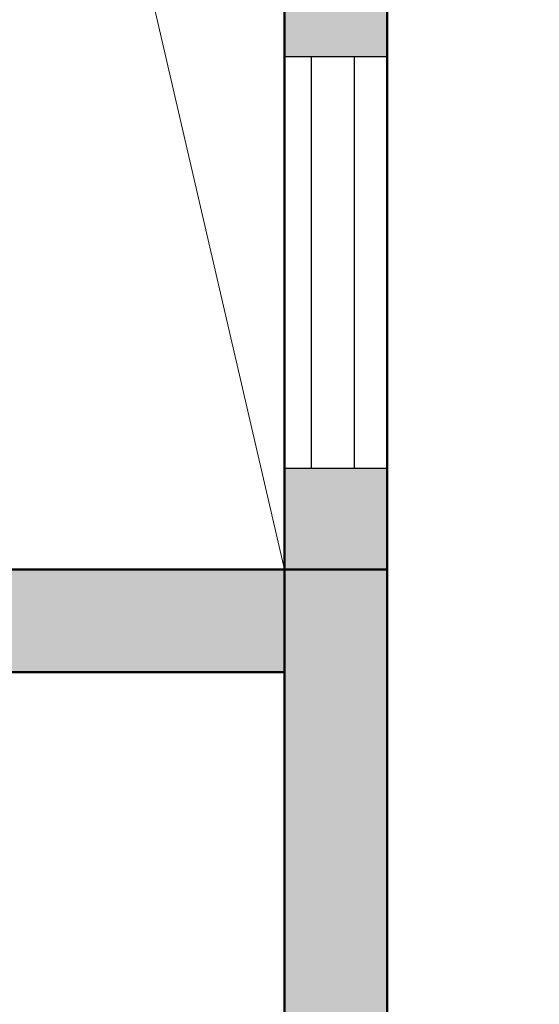
# Model space of a CAD drawing. Units: inches. Extents: x -7 to 1228, y -146 to 1091.
# Tile 67 of 88: x 611 to 656, y 617 to 703. Entities that reach past the tile are written whole.
import ezdxf

# ---------------------------------------------------------------- set-up
doc = ezdxf.new("R2010")
doc.units = ezdxf.units.IN
for name, color, linetype, lineweight in [('A-FLOR-VOID', 7, 'Continuous', 18), ('A-GLAZ', 175, 'Continuous', 25), ('A-WALL', 7, 'Continuous', 50), ('A-WALL-PATT', 251, 'Continuous', 13)]:
    doc.layers.add(name, color=color, linetype=linetype, lineweight=lineweight)

# ---------------------------------------------------------------- blocks, each defined once
blk = doc.blocks.new('WIN-36')
for p, q in [((0, 36), (0, 0)), ((9, 36), (0, 36)), ((2.343, 36), (2.343, 0)), ((6.137, 0), (6.137, 36)), ((9, 0), (9, 36)), ((0, 0), (9, 0)), ((2.343, 0), (6.137, 0))]:
    blk.add_line(p, q)

msp = doc.modelspace()

# ---------------------------------------------------------------- hatches: boundary and pattern name
at = {"layer": 'A-WALL-PATT'}
h = msp.add_hatch(color=256, dxfattribs=at)
h.dxf.hatch_style = 1
h.paths.add_polyline_path([(69, 568), (60, 568), (60, 493), (63.289, 493), (69, 493)])
h.paths.add_polyline_path([(69, 662.405), (60, 662.405), (60, 586), (69, 586)], flags=17)
h.paths.add_polyline_path([(69, 723), (184, 723), (184, 734), (179, 734), (179, 728), (69, 728), (69, 741.623), (60, 741.623), (60, 698.405), (69, 698.405)], flags=17)
h.paths.add_polyline_path([(69, 782), (231, 782), (231, 728), (231, 723), (231, 586), (236, 586), (236, 787), (69, 787), (69, 800.126), (60, 800.126), (60, 765.623), (69, 765.623)])
h.paths.add_polyline_path([(184, 842), (189, 842), (189, 848), (173, 848), (173, 842), (179, 842), (179, 787), (184, 787)])
h.paths.add_polyline_path([(118.22, 69), (69, 69), (69, 60), (118.22, 60)])
h.paths.add_polyline_path([(227, 69), (154.22, 69), (154.22, 60), (227, 60)])
h.paths.add_polyline_path([(236, 60), (232.711, 60), (227, 60), (227, 36), (236, 36)])
h.paths.add_polyline_path([(389, 60), (380, 60), (380, 36), (389, 36)])
h.paths.add_polyline_path([(384, 181), (380, 181), (380, 115), (380, 78), (384, 78)])
h.paths.add_polyline_path([(380, 115), (334.547, 115), (334.547, 109), (380, 109)])
h.paths.add_polyline_path([(274.547, 115), (236, 115), (236, 201), (232.711, 201), (231, 201), (231, 78), (236, 78), (236, 109), (274.547, 109)])
h.paths.add_polyline_path([(69, 123), (60, 123), (60, 78), (69, 78)])
h.paths.add_polyline_path([(69, 201), (60, 201), (60, 159), (69, 159)])
h.paths.add_polyline_path([(143, 219), (69, 219), (69, 213), (143, 213)], flags=17)
h.paths.add_polyline_path([(189, 219), (184, 219), (184, 274), (231, 274), (231, 219), (236, 219), (236, 279), (184, 279), (184, 297), (179, 297), (179, 279), (69, 279), (69, 290.912), (60, 290.912), (60, 262.179), (69, 262.179), (69, 274), (179, 274), (179, 219), (173, 219), (173, 213), (189, 213)])
h.paths.add_polyline_path([(69, 238.179), (60, 238.179), (60, 219), (69, 219)], flags=17)
h.paths.add_polyline_path([(69, 333), (60, 333), (60, 314.912), (69, 314.912), (69, 316.965)])
h.paths.add_polyline_path([(190, 338), (184, 338), (69, 338), (69, 333), (179, 333), (179, 327), (184, 327), (184, 333.021), (190, 333.046)])
h.paths.add_polyline_path([(69, 386.806), (60, 386.806), (60, 351), (69, 351)])
h.paths.add_polyline_path([(69, 475), (60, 475), (60, 422.806), (69, 422.806)])
h.paths.add_polyline_path([(236, 475), (231, 475), (231, 351.238), (236, 351.238)])
h.paths.add_polyline_path([(384, 475), (380, 475), (380, 362), (384, 362)])
h.paths.add_polyline_path([(547, 307), (439, 307), (439, 356), (445, 356), (445, 362), (433, 362), (433, 307), (380, 307), (380, 244), (380, 241), (384, 241), (384, 301), (433, 301), (433, 277), (439, 277), (439, 301), (547, 301)])
h.paths.add_polyline_path([(547, 241), (439, 241), (439, 247), (433, 247), (433, 235), (547, 235)])
h.paths.add_polyline_path([(450, 69), (440.286, 69), (424.889, 69), (389, 69), (389, 60), (450, 60)])
h.paths.add_polyline_path([(547, 69), (486, 69), (486, 60), (547, 60)])
h.paths.add_polyline_path([(556, 148.268), (547, 148.268), (547, 78), (556, 78)])
h.paths.add_polyline_path([(556, 223), (547, 223), (547, 195), (547, 184.268), (556, 184.268)])
h.paths.add_polyline_path([(556, 311.192), (547, 311.192), (547, 273.075), (556, 273.075)])
h.paths.add_polyline_path([(556, 344), (552.711, 344), (547, 344), (547, 335.192), (556, 335.192)])
h.paths.add_polyline_path([(556, 249.075), (547, 249.075), (547, 241), (556, 241)])
h.paths.add_polyline_path([(547, 362), (475, 362), (475, 356), (547, 356)], flags=0)
h.paths.add_polyline_path([(556, 399.621), (547, 399.621), (547, 362), (556, 362)])
h.paths.add_polyline_path([(556, 475), (547, 475), (547, 435.621), (556, 435.621)])
h.paths.add_polyline_path([(547, 493), (389, 493), (389, 487), (547, 487)])
h.paths.add_polyline_path([(380, 493), (278, 493), (278, 487), (380, 487)])
h.paths.add_polyline_path([(227, 493), (69, 493), (69, 487), (227, 487)])
h.paths.add_polyline_path([(643, 122.445), (634, 122.445), (634, 78), (643, 78)])
h.paths.add_polyline_path([(702.5, 69), (692.786, 69), (677.389, 69), (643, 69), (643, 60), (702.5, 60)])
h.paths.add_polyline_path([(798, 69), (738.5, 69), (738.5, 60), (798, 60)])
h.paths.add_polyline_path([(807, 60), (803.711, 60), (798, 60), (798, 36), (807, 36)])
h.paths.add_polyline_path([(807, 109), (846.751, 109), (846.751, 115), (807, 115), (807, 159), (802, 159), (802, 78), (807, 78)])
h.paths.add_polyline_path([(807, 201), (802, 201), (802, 195), (807, 195)])
h.paths.add_polyline_path([(643, 201), (634, 201), (634, 158.445), (643, 158.445)])
h.paths.add_polyline_path([(756, 225), (751, 225), (751, 219), (643, 219), (643, 213), (756, 213)])
h.paths.add_polyline_path([(643, 240.848), (634, 240.848), (634, 219), (643, 219)])
h.paths.add_polyline_path([(643, 274), (643, 288.629), (634, 288.629), (634, 264.848), (643, 264.848)])
h.paths.add_polyline_path([(802, 279), (756, 279), (756, 297), (751, 297), (751, 279), (643, 279), (643, 274), (751, 274), (751, 255), (756, 255), (756, 274), (802, 274)])
h.paths.add_polyline_path([(807, 333), (803.711, 333), (802, 333), (802, 279), (802, 274), (802, 219), (807, 219)])
h.paths.add_polyline_path([(956, 182), (951, 182), (951, 115), (906.751, 115), (906.751, 109), (951, 109), (951, 78), (956, 78)])
h.paths.add_polyline_path([(960, 60), (951, 60), (951, 36), (960, 36)])
h.paths.add_polyline_path([(1021, 69), (1005.781, 69), (960, 69), (960, 60), (1021, 60)])
h.paths.add_polyline_path([(956, 224), (951, 224), (951, 218), (956, 218)])
h.paths.add_polyline_path([(956, 302), (1004, 302), (1004, 278), (1010, 278), (1010, 302), (1118, 302), (1118, 290.809), (1127, 290.809), (1127, 326.968), (1118, 326.968), (1118, 320.966), (1118, 307), (1010, 307), (1010, 356), (1016, 356), (1016, 362), (1004, 362), (1004, 307), (951, 307), (951, 244), (951, 242), (954.289, 242), (956, 242)])
h.paths.add_polyline_path([(643, 333), (634, 333), (634, 312.629), (643, 312.629), (643, 316.965)])
h.paths.add_polyline_path([(756, 338), (643, 338), (643, 333), (751, 333), (751, 327), (756, 327)])
h.paths.add_polyline_path([(643, 388), (634, 388), (634, 351), (643, 351)])
h.paths.add_polyline_path([(807, 357), (802, 357), (802, 351), (807, 351)])
h.paths.add_polyline_path([(807, 475), (802, 475), (802, 393), (807, 393)])
h.paths.add_polyline_path([(643, 475), (634, 475), (634, 424), (643, 424)])
h.paths.add_polyline_path([(798, 493), (643, 493), (643, 487), (798, 487)])
h.paths.add_polyline_path([(634, 493), (556, 493), (556, 487), (634, 487)])
h.paths.add_polyline_path([(813, 493), (807, 493), (807, 487), (813, 487)])
h.paths.add_polyline_path([(951, 493), (849, 493), (849, 487), (951, 487)])
h.paths.add_polyline_path([(956, 484), (951, 484), (951, 374), (956, 374)])
h.paths.add_polyline_path([(1109, 493), (969, 493), (969, 487), (1109, 487)])
h.paths.add_polyline_path([(1127, 484), (1118, 484), (1118, 450.641), (1127, 450.641)])
h.paths.add_polyline_path([(1127, 414.641), (1118, 414.641), (1118, 365), (1127, 365)])
h.paths.add_polyline_path([(1109, 362), (1046, 362), (1046, 356), (1109, 356)], flags=17)
h.paths.add_polyline_path([(1127, 356), (1123.454, 356), (1118, 356), (1118, 350.968), (1127, 350.968)], flags=0)
h.paths.add_polyline_path([(1127, 266.809), (1118, 266.809), (1118, 262.361), (1118, 242), (1127, 242)], flags=17)
h.paths.add_polyline_path([(1118, 242), (1010, 242), (1010, 248), (1004, 248), (1004, 237), (1118, 237)])
h.paths.add_polyline_path([(1127, 224), (1118, 224), (1118, 170), (1127, 170)])
h.paths.add_polyline_path([(1127, 134), (1118, 134), (1118, 78), (1127, 78)])
h.paths.add_polyline_path([(1118, 69), (1057, 69), (1057, 60), (1118, 60)])
h.paths.add_polyline_path([(227, 571.546), (227, 574), (69, 574), (69, 568), (227, 568)])
h.paths.add_polyline_path([(380, 571.546), (380, 574), (278, 574), (278, 568), (380, 568)])
h.paths.add_polyline_path([(242, 574), (236, 574), (236, 568), (242, 568)])
h.paths.add_polyline_path([(547, 571.546), (547, 574), (389, 574), (389, 568), (547, 568)])
h.paths.add_polyline_path([(384, 733), (380, 733), (380, 586), (384, 586)])
h.paths.add_polyline_path([(556, 646), (634, 646), (634, 655), (547, 655), (547, 586), (556, 586)])
h.paths.add_polyline_path([(634, 574), (556, 574), (556, 568), (634, 568)])
h.paths.add_polyline_path([(643, 655), (634, 655), (634, 586), (643, 586)])
h.paths.add_polyline_path([(798, 574), (643, 574), (643, 568), (798, 568)])
h.paths.add_polyline_path([(643, 663.854), (634, 663.854), (634, 655), (643, 655)])
h.paths.add_polyline_path([(556, 676.967), (547, 676.967), (547, 655), (556, 655)])
h.paths.add_polyline_path([(556, 733), (547, 733), (547, 712.967), (556, 712.967)])
h.paths.add_polyline_path([(643, 710), (634, 710), (634, 699.854), (643, 699.854)])
h.paths.add_polyline_path([(807, 668), (802, 668), (802, 586), (807, 586)])
h.paths.add_polyline_path([(951, 574), (849, 574), (849, 568), (951, 568)])
h.paths.add_polyline_path([(956, 691), (951, 691), (951, 577), (956, 577)])
h.paths.add_polyline_path([(1109, 574), (969, 574), (969, 568), (1109, 568)])
h.paths.add_polyline_path([(1127, 643.403), (1118, 643.403), (1118, 577), (1127, 577)])
h.paths.add_polyline_path([(1127, 568), (1123.454, 568), (1118, 568), (1118, 493), (1127, 493)])
h.paths.add_polyline_path([(1127, 733), (1118, 733), (1118, 679.403), (1127, 679.403)])
h.paths.add_polyline_path([(1127, 777.348), (1118, 777.348), (1118, 770.035), (1118, 751), (1127, 751)], flags=17)
h.paths.add_polyline_path([(1118, 751), (1010, 751), (1010, 757), (1004, 757), (1004, 745), (1118, 745)])
h.paths.add_polyline_path([(956, 811), (1004, 811), (1004, 787), (1010, 787), (1010, 811), (1017.874, 811), (1017.874, 811.627, -0.414214), (1018.247, 812), (1031.978, 812, -0.414214), (1032.351, 811.627), (1032.351, 811), (1118, 811), (1118, 801.348), (1127, 801.348), (1127, 834.685), (1118, 834.685), (1118, 830.238), (1118, 817), (1010, 817), (1010, 866), (1016, 866), (1016, 872), (1004, 872), (1004, 817), (956, 817), (956, 866), (951, 866), (951, 751), (954.289, 751), (956, 751)])
h.paths.add_polyline_path([(1118, 872), (1046, 872), (1046, 866), (1118, 866)], flags=17)
h.paths.add_polyline_path([(1127, 924.711), (1118, 924.711), (1118, 884), (1127, 884)])
h.paths.add_polyline_path([(1127, 866), (1123.711, 866), (1118, 866), (1118, 858.685), (1127, 858.685)], flags=17)
h.paths.add_polyline_path([(956, 983), (951, 983), (951, 952), (807, 952), (807, 983), (802, 983), (802, 902), (807, 902), (807, 946), (951, 946), (951, 884), (956, 884)])
h.paths.add_polyline_path([(807, 842), (802, 842), (802, 787), (756, 787), (756, 806), (751, 806), (751, 787), (643, 787), (643, 782), (751, 782), (751, 764), (756, 764), (756, 782), (802, 782), (802, 728), (807, 728)])
h.paths.add_polyline_path([(756, 848), (643, 848), (643, 842), (751, 842), (751, 836), (756, 836)])
h.paths.add_polyline_path([(756, 734), (751, 734), (751, 728), (643, 728), (643, 723), (756, 723)])
h.paths.add_polyline_path([(643, 749.791), (634, 749.791), (634, 728), (637.289, 728), (643, 728)])
h.paths.add_polyline_path([(643, 805.405), (634, 805.405), (634, 773.791), (643, 773.791)])
h.paths.add_polyline_path([(643, 896.663), (634, 896.663), (634, 860), (637.289, 860), (643, 860)])
h.paths.add_polyline_path([(643, 842), (634, 842), (634, 829.405), (643, 829.405)])
h.paths.add_polyline_path([(643, 983), (634, 983), (634, 932.663), (643, 932.663)])
h.paths.add_polyline_path([(1127, 983), (1118, 983), (1118, 960.711), (1127, 960.711)])
h.paths.add_polyline_path([(1118, 1001), (1077.525, 1001), (1077.525, 992), (1118, 992)])
h.paths.add_polyline_path([(1041.525, 1001), (960, 1001), (960, 992), (1041.525, 992)])
h.paths.add_polyline_path([(960, 1025), (951, 1025), (951, 1001), (954.289, 1001), (960, 1001)])
h.paths.add_polyline_path([(807, 1025), (798, 1025), (798, 1001), (807, 1001)])
h.paths.add_polyline_path([(798, 1001), (738.5, 1001), (738.5, 992), (798, 992)])
h.paths.add_polyline_path([(702.5, 1001), (643, 1001), (643, 992), (702.5, 992)])
h.paths.add_polyline_path([(547, 1001), (499.113, 1001), (499.113, 992), (547, 992)])
h.paths.add_polyline_path([(463.113, 1001), (389, 1001), (389, 992), (463.113, 992)])
h.paths.add_polyline_path([(389, 1025), (380, 1025), (380, 1022), (380, 1001), (383.289, 1001), (389, 1001)])
h.paths.add_polyline_path([(236, 1025), (227, 1025), (227, 1001), (236, 1001)])
h.paths.add_polyline_path([(236, 983), (231, 983), (231, 860), (236, 860)])
h.paths.add_polyline_path([(274.547, 952), (236, 952), (236, 946), (274.547, 946)])
h.paths.add_polyline_path([(380, 952), (334.547, 952), (334.547, 946), (380, 946)])
h.paths.add_polyline_path([(384, 983), (380, 983), (380, 884), (383.289, 884), (384, 884)])
h.paths.add_polyline_path([(227, 1001), (155.012, 1001), (155.012, 992), (162.875, 992), (227, 992)])
h.paths.add_polyline_path([(119.012, 1001), (69, 1001), (69, 992), (119.012, 992)])
h.paths.add_polyline_path([(69, 983), (60, 983), (60, 922.987), (69, 922.987)])
h.paths.add_polyline_path([(69, 886.987), (60, 886.987), (60, 860), (63.289, 860), (69, 860)])
h.paths.add_polyline_path([(143, 848), (69, 848), (69, 842), (143, 842)])

# ---------------------------------------------------------------- linework, layer by layer
at = {"layer": 'A-FLOR-VOID'}
msp.add_line((556, 992), (634, 655), dxfattribs=at)
at = {"layer": 'A-WALL'}
for p, q in [((634, 1001), (634, 655)), ((634, 568), (634, 1001)), ((643, 568), (643, 1001)), ((643, 723), (643, 568)), ((643, 655), (547, 655)), ((634, 646), (556, 646)), ((634, 646), (634, 568))]:
    msp.add_line(p, q, dxfattribs=at)

# ---------------------------------------------------------------- block references
at = {"layer": 'A-GLAZ'}
msp.add_blockref('WIN-36', (634, 663.853), dxfattribs=at)

doc.saveas('drawing.dxf')
